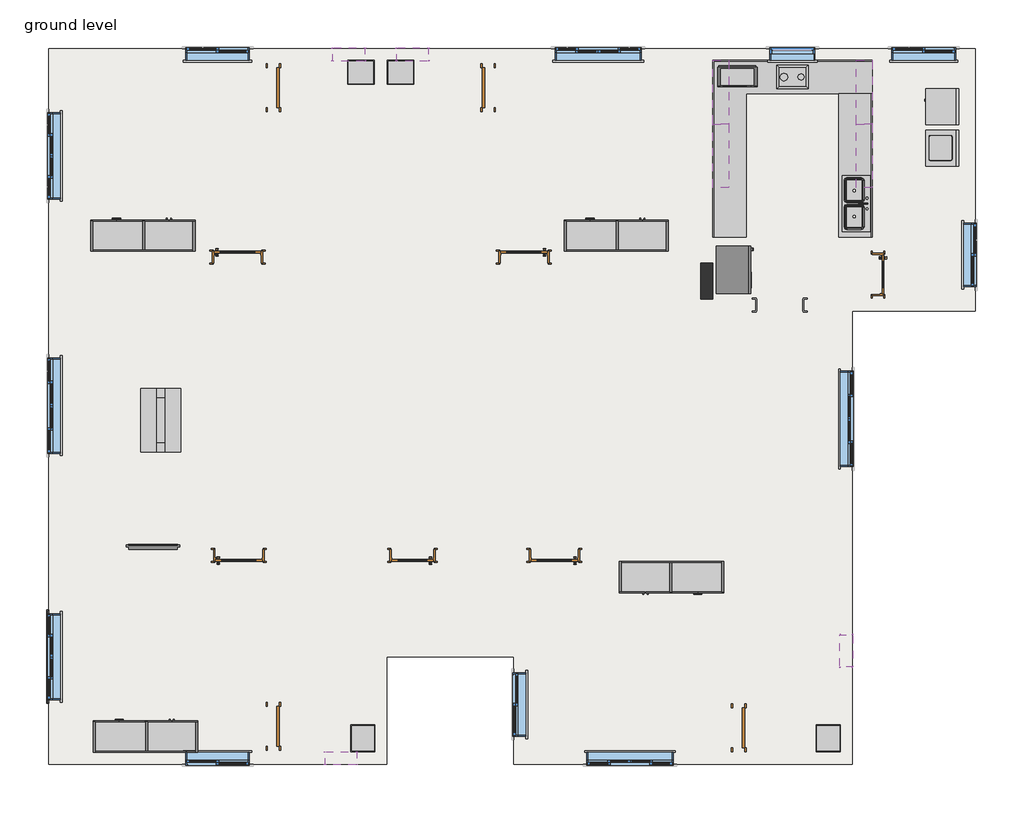
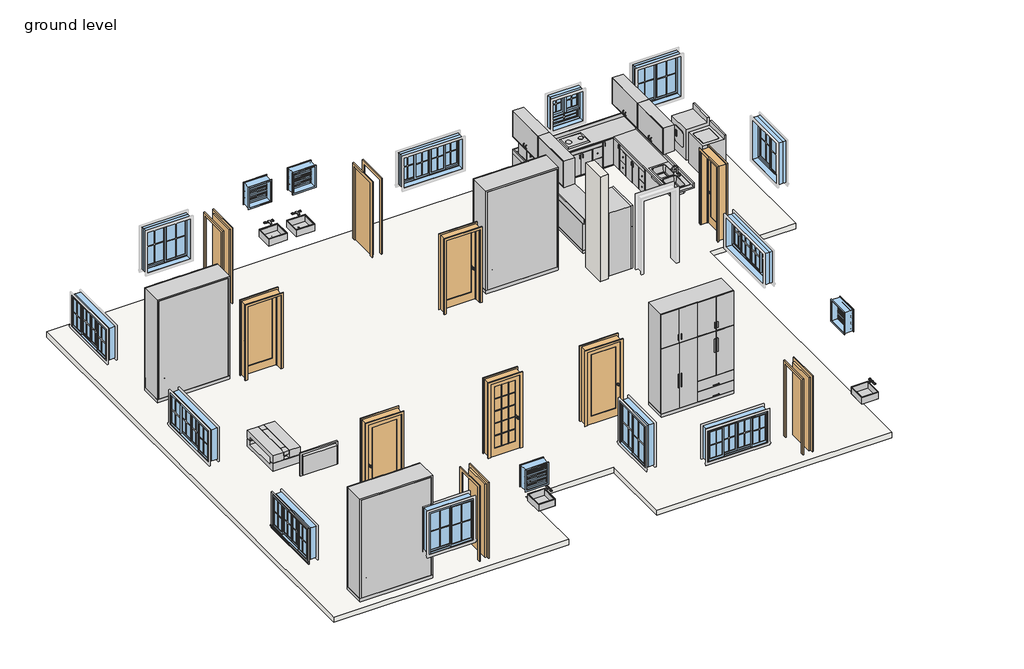
# One storey, part 1 of 2: 19 furniture elements, 16 windows, 10 doors, 10 proxies, 5 flow terminals, 1 slab, 1 wall.
"""IFC4 building model written with IfcOpenShell, lengths in millimetres."""

from ifc_helpers import new_model, si_unit, frame, origin, place, context, project, spatial, polyline, outline, extrude, transform, mapped, element, save
from components import proxy_3c1fa1d0, proxy_97c73763, proxy_e661f726, muntin_pattern_2x2_muntin_pattern_2x2_6186d23a, muntin_pattern_2x2_muntin_pattern_2x2_31a16349, muntin_pattern_2x2_muntin_pattern_2x2_cf37b409, trim_window_exterior_flat_with_sill_c3f87112, proxy_e75280ca, door_ac3c0746, door_868ee8a9, door_3b97b8e7, door_c0815308, door_5e1232af, door_bb98abfd, flow_terminal_cce4e9d2, flow_terminal_a53be723, furniture_65fa61b5, furniture_1wardrobe_6271_1wardrobe_6271_4dd35231, furniture_3428e43d, furniture_97fe820d, furniture_803bf5e8, furniture_2797bbf7, furniture_b6aab1a0, furniture_ea954fa4, white_modern_coffee_table_17067_white_modern_coffee_table_d4aed9ff, window_ced37e8f, window_f2d8fef0, window_5af5dca6, window_95c4569f, window_58cce754

model = new_model("IFC4")

# Units and contexts
model_context = context("Model", 3, world=origin())
ifc_project = project(units=[si_unit("LENGTHUNIT", "METRE", prefix="MILLI")], contexts=[model_context])

# Site, building, storey
site = spatial("IfcSite", under=ifc_project)
building = spatial("IfcBuilding", under=site)
storey = spatial("IfcBuildingStorey", under=building, Name="ground level", Elevation=609.6)

# Proxies
placement = place(None, origin())
proxy_shape = proxy_3c1fa1d0(model_context)
element("IfcBuildingElementProxy", 1, Name="Cook Top-2 Unit : 12\" x 18\" 2", ObjectType="Cook Top-2 Unit : 12\" x 18\" 2", at=placement, inside=storey, context=model_context, shape_type="MappedRepresentation", body=[
    mapped(proxy_shape, transform((6250.0508793, 6451.6660813, 609.6), x_axis=(0.0, 1.0, 0.0), y_axis=(-1.0, 0.0, 0.0), z_axis=(0.0, 0.0, 1.0))),
])
proxy_2_shape = proxy_97c73763(model_context)
element("IfcBuildingElementProxy", 2, Name="Dryer : 27\" x 25\" x 35\"", ObjectType="Dryer : 27\" x 25\" x 35\"", at=placement, inside=storey, context=model_context, shape_type="MappedRepresentation", body=[
    mapped(proxy_2_shape, transform((8776.0370876, 6339.378625, 609.6), x_axis=(0.0, -1.0, 0.0), y_axis=(1.0, 0.0, 0.0), z_axis=(0.0, 0.0, 1.0))),
])
proxy_3_shape = proxy_e661f726(model_context)
element("IfcBuildingElementProxy", 3, Name="Microwave : 30\" x 16\" x 18\"", ObjectType="Microwave : 30\" x 16\" x 18\"", at=placement, inside=storey, context=model_context, shape_type="MappedRepresentation", body=[
    mapped(proxy_3_shape, transform((4665.4332064, 6893.6465872, 609.6), x_axis=(1.0, 0.0, 0.0), y_axis=(0.0, 1.0, 0.0), z_axis=(0.0, 0.0, 1.0))),
])
muntin_pattern_2x2_muntin_pattern_2x2_shape = muntin_pattern_2x2_muntin_pattern_2x2_6186d23a(model_context)
element("IfcBuildingElementProxy", 4, Name="Muntin Pattern_2x2 : Muntin Pattern_2x2", ObjectType="Muntin Pattern_2x2 : Muntin Pattern_2x2", at=placement, inside=storey, context=model_context, shape_type="MappedRepresentation", body=[
    mapped(muntin_pattern_2x2_muntin_pattern_2x2_shape, transform((-8020.0489162, -5178.3589187, 1606.55), x_axis=(0.0, 1.0, 0.0), y_axis=(-1.0, 0.0, 0.0), z_axis=(0.0, 0.0, 1.0))),
])
element("IfcBuildingElementProxy", 5, Name="Muntin Pattern_2x2 : Muntin Pattern_2x2", ObjectType="Muntin Pattern_2x2 : Muntin Pattern_2x2", at=placement, inside=storey, context=model_context, shape_type="MappedRepresentation", body=[
    mapped(muntin_pattern_2x2_muntin_pattern_2x2_shape, transform((-8020.0489162, -3990.9089187, 1606.55), x_axis=(0.0, 1.0, 0.0), y_axis=(-1.0, 0.0, 0.0), z_axis=(0.0, 0.0, 1.0))),
])
muntin_pattern_2x2_muntin_pattern_2x2_2_shape = muntin_pattern_2x2_muntin_pattern_2x2_31a16349(model_context)
element("IfcBuildingElementProxy", 6, Name="Muntin Pattern_2x2 : Muntin Pattern_2x2", ObjectType="Muntin Pattern_2x2 : Muntin Pattern_2x2", at=placement, inside=storey, context=model_context, shape_type="MappedRepresentation", body=[
    mapped(muntin_pattern_2x2_muntin_pattern_2x2_2_shape, transform((-8020.0489162, -431.7339187, 1606.55), x_axis=(0.0, 1.0, 0.0), y_axis=(-1.0, 0.0, 0.0), z_axis=(0.0, 0.0, 1.0))),
])
muntin_pattern_2x2_muntin_pattern_2x2_3_shape = muntin_pattern_2x2_muntin_pattern_2x2_cf37b409(model_context)
element("IfcBuildingElementProxy", 7, Name="Muntin Pattern_2x2 : Muntin Pattern_2x2", ObjectType="Muntin Pattern_2x2 : Muntin Pattern_2x2", at=placement, inside=storey, context=model_context, shape_type="MappedRepresentation", body=[
    mapped(muntin_pattern_2x2_muntin_pattern_2x2_3_shape, transform((-5075.2364162, -6588.0589187, 1606.55), x_axis=(-1.0, 0.0, 0.0), y_axis=(0.0, -1.0, 0.0), z_axis=(0.0, 0.0, 1.0))),
])
element("IfcBuildingElementProxy", 8, Name="Muntin Pattern_2x2 : Muntin Pattern_2x2", ObjectType="Muntin Pattern_2x2 : Muntin Pattern_2x2", at=placement, inside=storey, context=model_context, shape_type="MappedRepresentation", body=[
    mapped(muntin_pattern_2x2_muntin_pattern_2x2_3_shape, transform((-4506.9114162, -6632.5089187, 1606.55), x_axis=(-1.0, 0.0, 0.0), y_axis=(0.0, -1.0, 0.0), z_axis=(0.0, 0.0, 1.0))),
])
trim_window_exterior_flat_with_sill_shape = trim_window_exterior_flat_with_sill_c3f87112(model_context)
element("IfcBuildingElementProxy", 9, Name="Trim-Window-Exterior-Flat : with Sill", ObjectType="Trim-Window-Exterior-Flat : with Sill", at=placement, inside=storey, context=model_context, shape_type="MappedRepresentation", body=[
    mapped(trim_window_exterior_flat_with_sill_shape, transform((-8029.5739162, -4584.6339187, 2438.4), x_axis=(0.0, -1.0, 0.0), y_axis=(0.0, 0.0, 1.0), z_axis=(-1.0, 0.0, 0.0))),
])
proxy_4_shape = proxy_e75280ca(model_context)
element("IfcBuildingElementProxy", 10, Name="Washer : 27\" x 25\" x 35\"", ObjectType="Washer : 27\" x 25\" x 35\"", at=placement, inside=storey, context=model_context, shape_type="MappedRepresentation", body=[
    mapped(proxy_4_shape, transform((8810.3756486, 5586.7486128, 609.6), x_axis=(0.0, -1.0, 0.0), y_axis=(1.0, 0.0, 0.0), z_axis=(0.0, 0.0, 1.0))),
])

# Doors
door_shape = door_ac3c0746(model_context)
element("IfcDoor", 11, ObjectType="Door-Interior-Single-1_Panel-Wood : 30\" x 84\"", at=placement, inside=storey, context=model_context, shape_type="MappedRepresentation", body=[
    mapped(door_shape, transform((7861.3010838, 2743.2660813, 609.6), x_axis=(0.0, -1.0, 0.0), y_axis=(1.0, 0.0, 0.0), z_axis=(0.0, 0.0, 1.0))),
])
door_2_shape = door_868ee8a9(model_context)
element("IfcDoor", 12, ObjectType="Door-Interior-Single-1_Panel-Wood : 36\" x 84\"", at=placement, inside=storey, context=model_context, shape_type="MappedRepresentation", body=[
    mapped(door_2_shape, transform((1076.3260838, 3076.6410813, 609.6), x_axis=(-1.0, 0.0, 0.0), y_axis=(0.0, -1.0, 0.0), z_axis=(0.0, 0.0, 1.0))),
])
element("IfcDoor", 13, ObjectType="Door-Interior-Single-1_Panel-Wood : 36\" x 84\"", at=placement, inside=storey, context=model_context, shape_type="MappedRepresentation", body=[
    mapped(door_2_shape, transform((-4384.6739162, -2644.7089187, 609.6), x_axis=(1.0, 0.0, 0.0), y_axis=(0.0, 1.0, 0.0), z_axis=(0.0, 0.0, 1.0))),
])
door_3_shape = door_3b97b8e7(model_context)
element("IfcDoor", 14, ObjectType="Door-Interior-Single-1_Panel-Wood : 36\" x 84\"", at=placement, inside=storey, context=model_context, shape_type="MappedRepresentation", body=[
    mapped(door_3_shape, transform((1660.5260838, -2644.7089187, 609.6), x_axis=(-1.0, 0.0, 0.0), y_axis=(0.0, -1.0, 0.0), z_axis=(0.0, 0.0, 1.0))),
])
element("IfcDoor", 15, ObjectType="Door-Interior-Single-1_Panel-Wood : 36\" x 84\"", at=placement, inside=storey, context=model_context, shape_type="MappedRepresentation", body=[
    mapped(door_3_shape, transform((-4410.0739162, 3076.6410813, 609.6), x_axis=(1.0, 0.0, 0.0), y_axis=(0.0, 1.0, 0.0), z_axis=(0.0, 0.0, 1.0))),
])
door_4_shape = door_c0815308(model_context)
element("IfcDoor", 16, ObjectType="Door-Interior-Single-Full Glass-Wood : 32\" x 84\"", at=placement, inside=storey, context=model_context, shape_type="MappedRepresentation", body=[
    mapped(door_4_shape, transform((-1057.2739162, -2644.7089187, 609.6), x_axis=(-1.0, 0.0, 0.0), y_axis=(0.0, -1.0, 0.0), z_axis=(0.0, 0.0, 1.0))),
])
door_5_shape = door_5e1232af(model_context)
element("IfcDoor", 17, ObjectType="Single-Flush : 30\" x 84\"", at=placement, inside=storey, context=model_context, shape_type="MappedRepresentation", body=[
    mapped(door_5_shape, transform((-3724.2739162, 6324.6660813, 609.6), x_axis=(0.0, 1.0, 0.0), y_axis=(-1.0, 0.0, 0.0), z_axis=(0.0, 0.0, 1.0))),
])
door_6_shape = door_bb98abfd(model_context)
element("IfcDoor", 18, ObjectType="Single-Flush : 30\" x 84\"", at=placement, inside=storey, context=model_context, shape_type="MappedRepresentation", body=[
    mapped(door_6_shape, transform((390.5260838, 6324.6660813, 609.6), x_axis=(0.0, 1.0, 0.0), y_axis=(-1.0, 0.0, 0.0), z_axis=(0.0, 0.0, 1.0))),
])
element("IfcDoor", 19, ObjectType="Single-Flush : 30\" x 84\"", at=placement, inside=storey, context=model_context, shape_type="MappedRepresentation", body=[
    mapped(door_6_shape, transform((-3724.2739162, -5918.1339187, 609.6), x_axis=(0.0, -1.0, 0.0), y_axis=(1.0, 0.0, 0.0), z_axis=(0.0, 0.0, 1.0))),
])
element("IfcDoor", 20, ObjectType="Single-Flush : 30\" x 84\"", at=placement, inside=storey, context=model_context, shape_type="MappedRepresentation", body=[
    mapped(door_6_shape, transform((5191.1260838, -5943.5339187, 609.6), x_axis=(0.0, -1.0, 0.0), y_axis=(1.0, 0.0, 0.0), z_axis=(0.0, 0.0, 1.0))),
])

# Flow terminals
flow_terminal_shape = flow_terminal_cce4e9d2(model_context)
element("IfcFlowTerminal", 21, ObjectType="Sink - Work : 20\"x18\"", at=placement, inside=storey, context=model_context, shape_type="MappedRepresentation", body=[
    mapped(flow_terminal_shape, transform((-1285.8739162, 6845.3660813, 1524.0), x_axis=(1.0, 0.0, 0.0), y_axis=(0.0, 1.0, 0.0), z_axis=(0.0, 0.0, 1.0))),
])
element("IfcFlowTerminal", 22, ObjectType="Sink - Work : 20\"x18\"", at=placement, inside=storey, context=model_context, shape_type="MappedRepresentation", body=[
    mapped(flow_terminal_shape, transform((-2047.8739162, 6845.3660813, 1524.0), x_axis=(1.0, 0.0, 0.0), y_axis=(0.0, 1.0, 0.0), z_axis=(0.0, 0.0, 1.0))),
])
element("IfcFlowTerminal", 23, ObjectType="Sink - Work : 20\"x18\"", at=placement, inside=storey, context=model_context, shape_type="MappedRepresentation", body=[
    mapped(flow_terminal_shape, transform((-1781.1739162, -6146.7339187, 1524.0), x_axis=(0.0, -1.0, 0.0), y_axis=(1.0, 0.0, 0.0), z_axis=(0.0, 0.0, 1.0))),
])
element("IfcFlowTerminal", 24, ObjectType="Sink - Work : 20\"x18\"", at=placement, inside=storey, context=model_context, shape_type="MappedRepresentation", body=[
    mapped(flow_terminal_shape, transform((7134.2260838, -6146.7339187, 1524.0), x_axis=(0.0, -1.0, 0.0), y_axis=(1.0, 0.0, 0.0), z_axis=(0.0, 0.0, 1.0))),
])
flow_terminal_2_shape = flow_terminal_a53be723(model_context)
element("IfcFlowTerminal", 25, ObjectType="Sink Kitchen-Double : 42\" x 21\"", at=placement, inside=storey, context=model_context, shape_type="MappedRepresentation", body=[
    mapped(flow_terminal_2_shape, transform((7436.6806826, 4117.8553219, 609.6), x_axis=(0.0, -1.0, 0.0), y_axis=(1.0, 0.0, 0.0), z_axis=(0.0, 0.0, 1.0))),
])

# Furniture
furniture_shape = furniture_65fa61b5(model_context)
element("IfcFurniture", 26, at=placement, inside=storey, context=model_context, shape_type="MappedRepresentation", body=[
    mapped(furniture_shape, transform((4759.3260838, 3441.7660813, 609.6), x_axis=(0.0, 1.0, 0.0), y_axis=(-1.0, 0.0, 0.0), z_axis=(0.0, 0.0, 1.0))),
])
furniture_1wardrobe_6271_1wardrobe_6271_shape = furniture_1wardrobe_6271_1wardrobe_6271_4dd35231(model_context)
element("IfcFurniture", 27, ObjectType="1Wardrobe_6271 : 1Wardrobe_6271", at=placement, inside=storey, context=model_context, shape_type="MappedRepresentation", body=[
    mapped(furniture_1wardrobe_6271_1wardrobe_6271_shape, transform((-5222.8739162, 3187.7660813, 609.6), x_axis=(-1.0, 0.0, 0.0), y_axis=(0.0, -1.0, 0.0), z_axis=(0.0, 0.0, 1.0))),
])
element("IfcFurniture", 28, ObjectType="1Wardrobe_6271 : 1Wardrobe_6271", at=placement, inside=storey, context=model_context, shape_type="MappedRepresentation", body=[
    mapped(furniture_1wardrobe_6271_1wardrobe_6271_shape, transform((3844.9260838, 3187.7660813, 609.6), x_axis=(-1.0, 0.0, 0.0), y_axis=(0.0, -1.0, 0.0), z_axis=(0.0, 0.0, 1.0))),
])
element("IfcFurniture", 29, ObjectType="1Wardrobe_6271 : 1Wardrobe_6271", at=placement, inside=storey, context=model_context, shape_type="MappedRepresentation", body=[
    mapped(furniture_1wardrobe_6271_1wardrobe_6271_shape, transform((2905.1260838, -2755.8339187, 609.6), x_axis=(1.0, 0.0, 0.0), y_axis=(0.0, 1.0, 0.0), z_axis=(0.0, 0.0, 1.0))),
])
element("IfcFurniture", 30, ObjectType="1Wardrobe_6271 : 1Wardrobe_6271", at=placement, inside=storey, context=model_context, shape_type="MappedRepresentation", body=[
    mapped(furniture_1wardrobe_6271_1wardrobe_6271_shape, transform((-5172.0739162, -6413.4339187, 609.6), x_axis=(-1.0, 0.0, 0.0), y_axis=(0.0, -1.0, 0.0), z_axis=(0.0, 0.0, 1.0))),
])
furniture_2_shape = furniture_3428e43d(model_context)
element("IfcFurniture", 31, ObjectType="48\" 2", at=placement, inside=storey, context=model_context, shape_type="MappedRepresentation", body=[
    mapped(furniture_2_shape, transform((6128.9811238, 6845.3660813, 609.6), x_axis=(1.0, 0.0, 0.0), y_axis=(0.0, 1.0, 0.0), z_axis=(0.0, 0.0, 1.0))),
])
element("IfcFurniture", 32, ObjectType="48\" 2", at=placement, inside=storey, context=model_context, shape_type="MappedRepresentation", body=[
    mapped(furniture_2_shape, transform((7743.8260838, 5412.2110413, 609.6), x_axis=(0.0, -1.0, 0.0), y_axis=(1.0, 0.0, 0.0), z_axis=(0.0, 0.0, 1.0))),
])
element("IfcFurniture", 33, ObjectType="48\" 2", at=placement, inside=storey, context=model_context, shape_type="MappedRepresentation", body=[
    mapped(furniture_2_shape, transform((4695.8260838, 5230.5211213, 609.6), x_axis=(0.0, 1.0, 0.0), y_axis=(-1.0, 0.0, 0.0), z_axis=(0.0, 0.0, 1.0))),
])
element("IfcFurniture", 34, ObjectType="48\" 2", at=placement, inside=storey, context=model_context, shape_type="MappedRepresentation", body=[
    mapped(furniture_2_shape, transform((4695.8260838, 4011.3211213, 609.6), x_axis=(0.0, 1.0, 0.0), y_axis=(-1.0, 0.0, 0.0), z_axis=(0.0, 0.0, 1.0))),
])
furniture_3_shape = furniture_97fe820d(model_context)
element("IfcFurniture", 35, ObjectType="Base Cabinet-Corner Unit-Square : 36\"", at=placement, inside=storey, context=model_context, shape_type="MappedRepresentation", body=[
    mapped(furniture_3_shape, transform((7217.0883788, 6845.3660813, 609.6), x_axis=(1.0, 0.0, 0.0), y_axis=(0.0, 1.0, 0.0), z_axis=(0.0, 0.0, 1.0))),
])
element("IfcFurniture", 36, ObjectType="Base Cabinet-Corner Unit-Square : 36\"", at=placement, inside=storey, context=model_context, shape_type="MappedRepresentation", body=[
    mapped(furniture_3_shape, transform((4695.8260838, 6318.6283764, 609.6), x_axis=(0.0, 1.0, 0.0), y_axis=(-1.0, 0.0, 0.0), z_axis=(0.0, 0.0, 1.0))),
])
furniture_4_shape = furniture_803bf5e8(model_context)
element("IfcFurniture", 37, ObjectType="Counter Top w Sink : 24\" Depth", at=placement, inside=storey, context=model_context, shape_type="MappedRepresentation", body=[
    mapped(furniture_4_shape, transform((7743.8260838, 5009.9037862, 609.6), x_axis=(0.0, -1.0, 0.0), y_axis=(1.0, 0.0, 0.0), z_axis=(0.0, 0.0, 1.0))),
])
furniture_5_shape = furniture_2797bbf7(model_context)
element("IfcFurniture", 38, ObjectType="Counter Top-L Shaped : 24\" Depth", at=placement, inside=storey, context=model_context, shape_type="MappedRepresentation", body=[
    mapped(furniture_5_shape, transform((5896.2883788, 6845.3660813, 609.6), x_axis=(1.0, 0.0, 0.0), y_axis=(0.0, 1.0, 0.0), z_axis=(0.0, 0.0, 1.0))),
])
furniture_6_shape = furniture_b6aab1a0(model_context)
element("IfcFurniture", 39, ObjectType="Television-Plasma : 42\"", at=placement, inside=storey, context=model_context, shape_type="MappedRepresentation", body=[
    mapped(furniture_6_shape, transform((-5972.1739162, -2527.2339187, 1676.4), x_axis=(-1.0, 0.0, 0.0), y_axis=(0.0, -1.0, 0.0), z_axis=(0.0, 0.0, 1.0))),
])
furniture_7_shape = furniture_ea954fa4(model_context)
element("IfcFurniture", 40, ObjectType="Upper Cabinet-Pass-Thru : 48\" x 30\" x 12\"", at=placement, inside=storey, context=model_context, shape_type="MappedRepresentation", body=[
    mapped(furniture_7_shape, transform((4695.8260838, 6217.0283764, 609.6), x_axis=(0.0, 1.0, 0.0), y_axis=(-1.0, 0.0, 0.0), z_axis=(0.0, 0.0, 1.0))),
])
element("IfcFurniture", 41, ObjectType="Upper Cabinet-Pass-Thru : 48\" x 30\" x 12\"", at=placement, inside=storey, context=model_context, shape_type="MappedRepresentation", body=[
    mapped(furniture_7_shape, transform((4695.8260838, 4997.8283764, 609.6), x_axis=(0.0, 1.0, 0.0), y_axis=(-1.0, 0.0, 0.0), z_axis=(0.0, 0.0, 1.0))),
])
element("IfcFurniture", 42, ObjectType="Upper Cabinet-Pass-Thru : 48\" x 30\" x 12\"", at=placement, inside=storey, context=model_context, shape_type="MappedRepresentation", body=[
    mapped(furniture_7_shape, transform((7743.8260838, 6254.5037862, 609.6), x_axis=(0.0, -1.0, 0.0), y_axis=(1.0, 0.0, 0.0), z_axis=(0.0, 0.0, 1.0))),
])
element("IfcFurniture", 43, ObjectType="Upper Cabinet-Pass-Thru : 48\" x 30\" x 12\"", at=placement, inside=storey, context=model_context, shape_type="MappedRepresentation", body=[
    mapped(furniture_7_shape, transform((7743.8260838, 5035.3037862, 609.6), x_axis=(0.0, -1.0, 0.0), y_axis=(1.0, 0.0, 0.0), z_axis=(0.0, 0.0, 1.0))),
])
white_modern_coffee_table_17067_white_modern_coffee_table_shape = white_modern_coffee_table_17067_white_modern_coffee_table_d4aed9ff(model_context)
element("IfcFurniture", 44, ObjectType="White_Modern_Coffee_Table_17067 : White_Modern_Coffee_Table_17067", at=placement, inside=storey, context=model_context, shape_type="MappedRepresentation", body=[
    mapped(white_modern_coffee_table_17067_white_modern_coffee_table_shape, transform((-5878.4127262, -50.7339187, 609.6), x_axis=(0.0, 1.0, 0.0), y_axis=(-1.0, 0.0, 0.0), z_axis=(0.0, 0.0, 1.0))),
])

# Slab
element("IfcSlab", 45, ObjectType="Generic - 6\"", at=placement, inside=storey, context=model_context, shape_type="SweptSolid", body=[
    extrude(outline(polyline([(9725.2894662, 7073.9660813), (9725.2894662, 2044.7660813), (7362.8260838, 2044.7660813), (7362.8260838, -6642.0339187), (885.8260838, -6642.0339187), (885.8260838, -4584.6339187), (-1552.5739162, -4584.6339187), (-1552.5739162, -6642.0339187), (-8029.5739162, -6642.0339187), (-8029.5739162, 7073.9660813), (9725.2894662, 7073.9660813)])), frame((0.0, 0.0, 457.2), z_axis=(0.0, 0.0, 1.0), x_axis=(1.0, 0.0, 0.0)), (0.0, 0.0, 1.0), 152.4),
])

# Wall
element("IfcWall", 46, ObjectType="Generic - 9\"", at=placement, inside=storey, context=model_context, shape_type="SweptSolid", body=[
    extrude(outline(polyline([(4695.8260838, 2959.1660813), (4695.8260838, 2273.3660813), (4467.2260838, 2273.3660813), (4467.2260838, 2959.1660813), (4695.8260838, 2959.1660813)])), frame((0.0, 0.0, 609.6), z_axis=(0.0, 0.0, 1.0), x_axis=(1.0, 0.0, 0.0)), (0.0, 0.0, 1.0), 3048.0),
])

# Windows
window_shape = window_ced37e8f(model_context)
element("IfcWindow", 47, ObjectType="Window-Casement-Double-Awning : 34\" x 36\"", at=placement, inside=storey, context=model_context, shape_type="MappedRepresentation", body=[
    mapped(window_shape, transform((6219.8260838, 6959.6660813, 838.2), x_axis=(1.0, 0.0, 0.0), y_axis=(0.0, 1.0, 0.0), z_axis=(0.0, 0.0, 1.0))),
])
window_2_shape = window_f2d8fef0(model_context)
element("IfcWindow", 48, ObjectType="Window-Louvers : 24\" x 24\"", at=placement, inside=storey, context=model_context, shape_type="MappedRepresentation", body=[
    mapped(window_2_shape, transform((-2276.4739162, 6966.0160813, 1524.0), x_axis=(1.0, 0.0, 0.0), y_axis=(0.0, 1.0, 0.0), z_axis=(0.0, 0.0, 1.0))),
])
element("IfcWindow", 49, ObjectType="Window-Louvers : 24\" x 24\"", at=placement, inside=storey, context=model_context, shape_type="MappedRepresentation", body=[
    mapped(window_2_shape, transform((-1057.2739162, 6966.0160813, 1524.0), x_axis=(1.0, 0.0, 0.0), y_axis=(0.0, 1.0, 0.0), z_axis=(0.0, 0.0, 1.0))),
])
element("IfcWindow", 50, ObjectType="Window-Louvers : 24\" x 24\"", at=placement, inside=storey, context=model_context, shape_type="MappedRepresentation", body=[
    mapped(window_2_shape, transform((-2428.8739162, -6534.0839187, 1524.0), x_axis=(-1.0, 0.0, 0.0), y_axis=(0.0, -1.0, 0.0), z_axis=(0.0, 0.0, 1.0))),
])
element("IfcWindow", 51, ObjectType="Window-Louvers : 24\" x 24\"", at=placement, inside=storey, context=model_context, shape_type="MappedRepresentation", body=[
    mapped(window_2_shape, transform((7254.8760838, -4470.3339187, 1524.0), x_axis=(0.0, -1.0, 0.0), y_axis=(1.0, 0.0, 0.0), z_axis=(0.0, 0.0, 1.0))),
])
window_3_shape = window_5af5dca6(model_context)
element("IfcWindow", 52, ObjectType="Window-Sliding-Double : 48\" x 48\"", at=placement, inside=storey, context=model_context, shape_type="MappedRepresentation", body=[
    mapped(window_3_shape, transform((996.3160838, -5499.0339187, 609.6), x_axis=(0.0, 1.0, 0.0), y_axis=(-1.0, 0.0, 0.0), z_axis=(0.0, 0.0, 1.0))),
])
element("IfcWindow", 53, ObjectType="Window-Sliding-Double : 48\" x 48\"", at=placement, inside=storey, context=model_context, shape_type="MappedRepresentation", body=[
    mapped(window_3_shape, transform((8734.4260838, 6963.4760813, 609.6), x_axis=(1.0, 0.0, 0.0), y_axis=(0.0, 1.0, 0.0), z_axis=(0.0, 0.0, 1.0))),
])
element("IfcWindow", 54, ObjectType="Window-Sliding-Double : 48\" x 48\"", at=placement, inside=storey, context=model_context, shape_type="MappedRepresentation", body=[
    mapped(window_3_shape, transform((9614.7994662, 3116.7811041, 609.6), x_axis=(0.0, -1.0, 0.0), y_axis=(1.0, 0.0, 0.0), z_axis=(0.0, 0.0, 1.0))),
])
element("IfcWindow", 55, ObjectType="Window-Sliding-Double : 48\" x 48\"", at=placement, inside=storey, context=model_context, shape_type="MappedRepresentation", body=[
    mapped(window_3_shape, transform((-4791.0739162, -6531.5439187, 609.6), x_axis=(-1.0, 0.0, 0.0), y_axis=(0.0, -1.0, 0.0), z_axis=(0.0, 0.0, 1.0))),
])
element("IfcWindow", 56, ObjectType="Window-Sliding-Double : 48\" x 48\"", at=placement, inside=storey, context=model_context, shape_type="MappedRepresentation", body=[
    mapped(window_3_shape, transform((-4791.0739162, 6963.4760813, 609.6), x_axis=(1.0, 0.0, 0.0), y_axis=(0.0, 1.0, 0.0), z_axis=(0.0, 0.0, 1.0))),
])
window_4_shape = window_95c4569f(model_context)
element("IfcWindow", 57, ObjectType="Window-Sliding-Four : 65\" x 36\"", at=placement, inside=storey, context=model_context, shape_type="MappedRepresentation", body=[
    mapped(window_4_shape, transform((2498.7260838, 6963.4760813, 609.6), x_axis=(1.0, 0.0, 0.0), y_axis=(0.0, 1.0, 0.0), z_axis=(0.0, 0.0, 1.0))),
])
element("IfcWindow", 58, ObjectType="Window-Sliding-Four : 65\" x 36\"", at=placement, inside=storey, context=model_context, shape_type="MappedRepresentation", body=[
    mapped(window_4_shape, transform((3108.3260838, -6531.5439187, 609.6), x_axis=(-1.0, 0.0, 0.0), y_axis=(0.0, -1.0, 0.0), z_axis=(0.0, 0.0, 1.0))),
])
element("IfcWindow", 59, ObjectType="Window-Sliding-Four : 65\" x 36\"", at=placement, inside=storey, context=model_context, shape_type="MappedRepresentation", body=[
    mapped(window_4_shape, transform((-7919.0839162, 5016.5660813, 609.6), x_axis=(0.0, 1.0, 0.0), y_axis=(-1.0, 0.0, 0.0), z_axis=(0.0, 0.0, 1.0))),
])
element("IfcWindow", 60, ObjectType="Window-Sliding-Four : 65\" x 36\"", at=placement, inside=storey, context=model_context, shape_type="MappedRepresentation", body=[
    mapped(window_4_shape, transform((-7919.0839162, -4584.6339187, 609.6), x_axis=(0.0, 1.0, 0.0), y_axis=(-1.0, 0.0, 0.0), z_axis=(0.0, 0.0, 1.0))),
])
window_5_shape = window_58cce754(model_context)
element("IfcWindow", 61, ObjectType="Window-Sliding-Four : 72\" x 36\"", at=placement, inside=storey, context=model_context, shape_type="MappedRepresentation", body=[
    mapped(window_5_shape, transform((-7919.0839162, 228.6660813, 609.6), x_axis=(0.0, 1.0, 0.0), y_axis=(-1.0, 0.0, 0.0), z_axis=(0.0, 0.0, 1.0))),
])
element("IfcWindow", 62, ObjectType="Window-Sliding-Four : 72\" x 36\"", at=placement, inside=storey, context=model_context, shape_type="MappedRepresentation", body=[
    mapped(window_5_shape, transform((7252.3360838, -25.3339187, 609.6), x_axis=(0.0, -1.0, 0.0), y_axis=(1.0, 0.0, 0.0), z_axis=(0.0, 0.0, 1.0))),
])

save(model, "model.ifc")

# Revit data of these elements
# Type "Cook Top-2 Unit : 12\" x 18\" 2"
#   Assembly Code = "E1090400"
#   Counter Height = 3' - 0"
#   Depth = 2' - 0"
#   Width = 1' - 6"
#   Burner Material = Metal - Chrome
#   Cooktop Material = Metal - Steel, Polished
#   Default Elevation = 0
# Type "Dryer : 27\" x 25\" x 35\""
#   Label = "D"
#   Assembly Code = "E1090400"
#   Depth = 2' - 1"
#   Height = 2' - 11"
#   Width = 2' - 3"
#   Dryer Material = Metal - Paint Finish - Ivory,Glossy
#   Default Elevation = 0
# Type "Microwave : 30\" x 16\" x 18\""
#   Assembly Code = "E1090400"
#   Depth = 1' - 4"
#   Height = 1' - 6"
#   Width = 2' - 6"
#   Microwave Material = Laminate - Ivory,Matte
#   Default Elevation = 0
# Type "Muntin Pattern_2x2 : Muntin Pattern_2x2"
#   Width [instance default] = 4' - 0"
#   Thickness = 0' - 0 1/2"
#   Height [instance default] = 4' - 0"
#   Distance = 0' - 0 3/4"
#   Interior Material [instance default] = none
#   Exterior Material [instance default] = none
#   Default Elevation = 0
# Type "Trim-Window-Exterior-Flat : with Sill"
#   Trim Width = 0' - 2 1/4"
#   Trim Thickness_Picture Frame = 0' - 1 1/4"
#   Trim Thickness_with Sill = 0' - 0 3/4"
#   Sill Thickness = 0' - 1 1/4"
#   Opening Width [instance default] = 2' - 0"
#   Opening Height [instance default] = 3' - 0"
#   Default Elevation = 4' - 0"
#   Sill = yes
#   Picture Frame = no
#   Trim Material [instance default] = none
# Type "Washer : 27\" x 25\" x 35\""
#   Label = "W"
#   Assembly Code = "E1090400"
#   Depth = 2' - 1"
#   Height = 2' - 11"
#   Width = 2' - 3"
#   Washer Material = Metal - Paint Finish - Ivory,Matte
#   Default Elevation = 0
# Type "Door-Interior-Single-1_Panel-Wood : 30\" x 84\""
#   Type Mark = "11"
#   Assembly Code = "C1020300"
#   Analytic Construction = "Wooden"
#   Top Rail = 0' - 4 11/16"
#   Thickness = 0' - 1 3/8"
#   Thermal Resistance (R) = 2.5876 (h·ft²·°F)/BTU
#   Swing Angle [instance default] = 90.00°
#   Stiles = 0' - 4 3/4"
#   Rough Width = 2' - 8"
#   Rough Height = 7' - 1"
#   Height = 7' - 0"
#   Width = 2' - 6"
#   Heat Transfer Coefficient (U) = 0.3865 BTU/(h·ft²·°F)
#   Bottom Rail = 0' - 9 1/8"
#   Trim Material = Cherry
#   Panel Material = Cherry
#   Frame Material = Cherry
#   Door Handle Material = Aluminum
#   Visual Light Transmittance = 0
#   Solar Heat Gain Coefficient = 0
#   Wall Closure = (empty or 0)
#   Function = (empty or 0)
# Type "Door-Interior-Single-1_Panel-Wood : 36\" x 84\""
#   Type Mark = "8"
#   Assembly Code = "C1020300"
#   Analytic Construction = "Wooden"
#   Top Rail = 0' - 4 11/16"
#   Thickness = 0' - 1 3/8"
#   Thermal Resistance (R) = 2.5876 (h·ft²·°F)/BTU
#   Swing Angle [instance default] = 90.00°
#   Stiles = 0' - 4 3/4"
#   Rough Width = 3' - 2"
#   Rough Height = 7' - 1"
#   Height = 7' - 0"
#   Width = 3' - 0"
#   Heat Transfer Coefficient (U) = 0.3865 BTU/(h·ft²·°F)
#   Bottom Rail = 0' - 9 1/8"
#   Trim Material = Cherry
#   Panel Material = Cherry
#   Frame Material = Cherry
#   Door Handle Material = Aluminum
#   Visual Light Transmittance = 0
#   Solar Heat Gain Coefficient = 0
#   Wall Closure = (empty or 0)
#   Function = (empty or 0)
# Type "Door-Interior-Single-Full Glass-Wood : 32\" x 84\""
#   Type Mark = "9"
#   Assembly Code = "C1020300"
#   Analytic Construction = "Wood frame with single clear glass"
#   Top Rail = 0' - 4 11/16"
#   Thickness = 0' - 1 3/8"
#   Thermal Resistance (R) = 1.0102 (h·ft²·°F)/BTU
#   Swing Angle [instance default] = 90.00°
#   Stiles = 0' - 4 3/4"
#   Rough Width = 2' - 10"
#   Rough Height = 7' - 1"
#   Height = 7' - 0"
#   Width = 2' - 8"
#   Heat Transfer Coefficient (U) = 0.9900 BTU/(h·ft²·°F)
#   Bottom Rail = 0' - 9 1/8"
#   Show Grill [instance default] = yes
#   Trim Material = Cherry
#   Panel Material = Cherry
#   Frame Material = Cherry
#   Door Handle Material = Aluminum
#   Visual Light Transmittance = 0
#   Solar Heat Gain Coefficient = 0
#   Wall Closure = (empty or 0)
#   Function = (empty or 0)
# Type "Single-Flush : 30\" x 84\""
#   Type Mark = "4"
#   Construction Type Id = "MDOOR"
#   Assembly Code = "C1020"
#   Analytic Construction = "Metal"
#   Thickness = 0' - 2"
#   Heat Transfer Coefficient (U) = 0.651978 BTU/(h·ft²·°F)
#   Height = 7' - 0"
#   Trim Projection Ext = 0' - 1"
#   Trim Projection Int = 0' - 1"
#   Trim Width = 0' - 3"
#   Width = 2' - 6"
#   Define Thermal Properties by = 1
#   Define Thermal Properties by = 1
#   Door Material = Door - Panel
#   Frame Material = Door - Frame
#   Visual Light Transmittance = 0
#   Solar Heat Gain Coefficient = 0
#   Function = (empty or 0)
#   Wall Closure = (empty or 0)
# Type "Sink - Work : 20\"x18\""
#   WFU = 2
#   Sink Width = 1' - 6"
#   Sink Length = 1' - 8"
#   Sink Depth = 0' - 8"
#   Sanitary Radius = 3/4"
#   Sanitary Diameter = 1 1/2"
#   Hot Water Radius = 1/4"
#   Hot Water Diameter = 1/2"
#   HWFU = 2.25
#   Flow Pressure [instance default] = 8.00 psi
#   Faucet Height = 1' - 1 5/8"
#   Cold Water Radius = 1/4"
#   Cold Water Diameter = 1/2"
#   CWFU = 2.25
#   Sink Material = none
#   Faucet Material = none
#   Default Elevation = 0
# Type "Sink Kitchen-Double : 42\" x 21\""
#   Assembly Code = "D2010410"
#   Counter Height = 3' - 0"
#   Depth = 1' - 9"
#   Width = 3' - 6"
#   Faucet Material = Steel, Polished
#   Sink Material = Steel, Polished
#   Default Elevation = 0
# Type
#   Default Elevation = 0
# Type "1Wardrobe_6271 : 1Wardrobe_6271"
#   Default Elevation = 0
# Type "48\" 2"
#   Assembly Code = "C1030410"
#   Depth = 2' - 0"
#   Height = 2' - 10 1/2"
#   Toe Depth = 0' - 3"
#   Toe Height = 0' - 3 1/2"
#   Width = 4' - 0"
#   Cabinet Material = none
#   Door/Drawer Material = none
#   Handle Material = Cabinets - Handles
#   Default Elevation = 0
# Type "Base Cabinet-Corner Unit-Square : 36\""
#   Assembly Code = "C1030410"
#   Depth = 2' - 0"
#   Height = 2' - 10 1/2"
#   Toe Depth = 0' - 3"
#   Toe Height = 0' - 3 1/2"
#   Width = 3' - 0"
#   Cabinet Material = Cabinets
#   Door/Drawer Material = Cabinets
#   Handle Material = Cabinets - Handles
#   Default Elevation = 0
# Type "Counter Top w Sink : 24\" Depth"
#   Assembly Code = "C1030400"
#   Counter Thickness = 0' - 1 1/2"
#   Depth = 2' - 1"
#   Height = 3' - 0"
#   Length [instance default] = 8' - 0"
#   Sink Location [instance default] = 2' - 0"
#   Sink Location To Wall [instance default] = 0' - 6"
#   Sink Opening Depth [instance default] = 1' - 3"
#   Sink Opening Width [instance default] = 3' - 3"
#   Counter Top Material = none
#   Default Elevation = 0
# Type "Counter Top-L Shaped : 24\" Depth"
#   Assembly Code = "C1030400"
#   Counter Thickness = 0' - 1 1/2"
#   Depth = 2' - 1"
#   Height = 3' - 0"
#   Length - Leg 1 [instance default] = 8' - 0"
#   Length - Leg 2 [instance default] = 6' - 0"
#   Counter Top Material = none
#   Default Elevation = 0
# Type "Television-Plasma : 42\""
#   Assembly Code = "E2020200"
#   Depth = 0' - 3 1/2"
#   Height = 2' - 2"
#   Width = 3' - 4 1/2"
#   Cabinet Material = Plastic - Gray
#   Default Elevation = 0
# Type "Upper Cabinet-Pass-Thru : 48\" x 30\" x 12\""
#   Depth = 1' - 0"
#   Height = 2' - 6"
#   Top of Cabinet = 7' - 0"
#   Width = 4' - 0"
#   Default Elevation = 0
# Type "White_Modern_Coffee_Table_17067 : White_Modern_Coffee_Table_17067"
#   White Modern Coffee Table - Wood Width = 0' - 6"
#   White Modern Coffee Table - Width = 2' - 6"
#   White Modern Coffee Table - Length = 4' - 0"
#   White Modern Coffee Table - Wood = White Modern Coffee Table - Wood
#   White Modern Coffee Table - Plastic = White Modern Coffee Table - Plastic
#   Default Elevation = 0
# Type "Generic - 6\""
#   Assembly Code = "B1010"
#   Function = 0
#   Layers, outside or top first: 0' - 6" no material (function 1)
# Type "Generic - 9\""
#   Assembly Code = "B2010"
#   Layers, outside or top first: 0' - 9" no material (function 1)
# Type "Window-Casement-Double-Awning : 34\" x 36\""
#   Type Mark = "26"
#   Fire Rating = "0.5h"
#   Assembly Code = "B2020100"
#   Analytic Construction = "Double glazing - domestic"
#   Window Inset [instance default] = 0' - 0"
#   Wall Thickness [instance default] = 0' - 6"
#   Interior Wall Closure [instance default] = 0' - 2 1/4"
#   Half Width = 1' - 5"
#   Visual Light Transmittance = 0.81
#   Thermal Resistance (R) = 1.8146 (h·ft²·°F)/BTU
#   Solar Heat Gain Coefficient = 0.76
#   Rough Width = 2' - 10 1/2"
#   Rough Height = 3' - 0 1/2"
#   Open Window Height = 2' - 0"
#   Height = 3' - 0"
#   Heat Transfer Coefficient (U) = 0.5511 BTU/(h·ft²·°F)
#   Frame Extension [instance default] = 0' - 0 1/4"
#   Exterior Wall Closure [instance default] = 0' - 1 1/4"
#   Awning Height = 1' - 0"
#   Extension Jamb [instance default] = 0' - 2 1/4"
#   Default Sill Height = 3' - 0"
#   Width = 2' - 10"
#   Top Muntin Visibility = yes
#   Interior Trim Visibility [instance default] = yes
#   Bottom Muntin Visibility = yes
#   Exterior Trim Visibility [instance default] = yes
#   Extension Jamb Visibility [instance default] = yes
#   Interior Trim Material = Wood - Stained
#   Muntin Pattern = Muntin Pattern_2x2 : Muntin Pattern_2x2
#   Interior Trim = Trim-Window-Interior-Flat : Picture Frame
#   Interior Frame Material = Wood - Stained
#   Exterior Trim Material = Clad - White
#   Glass Panel Material = Glass
#   Exterior Trim = Trim-Window-Exterior-Flat : with Sill
#   Exterior Frame Material = Clad - White
#   Wall Closure = (empty or 0)
# Type "Window-Louvers : 24\" x 24\""
#   Type Mark = "24"
#   Construction Type Id = "GSP4R"
#   Assembly Code = "B20"
#   Analytic Construction = "1/8 in Pilkington single glazing"
#   Visual Light Transmittance = 0.9
#   Thermal Resistance (R) = 1.53941 (h·ft²·°F)/BTU
#   Solar Heat Gain Coefficient = 0.78
#   Max Height = 1' - 11.74264"
#   Height = 2' - 0"
#   Heat Transfer Coefficient (U) = 0.6496 BTU/(h·ft²·°F)
#   Blade Width [instance default] = 1' - 10 1/2"
#   Blade Vertical Thickness = 0' - 0.35355"
#   Blade Thickness = 0' - 0 1/4"
#   Blade Spacing = 0' - 1 1/2"
#   Blade Height = 0' - 1.85355"
#   Blade Depth = 0' - 3"
#   Blade Angle = 45.00°
#   Default Sill Height = 3' - 0"
#   Trim Projection_Exterior = 0' - 0 1/2"
#   Trim Projection_Interior = 0' - 0 1/2"
#   Trim Width_Exterior = 0' - 1 1/2"
#   Trim Width_Interior = 0' - 1 1/2"
#   Width = 2' - 0"
#   Max Blade Count = 12
#   Define Thermal Properties by = 1
#   Blade Count = 12
#   Frame Material = Birch
#   Louver Material = Birch
#   Trim Exterior Material = Birch
#   Trim Interior Material = Birch
#   Wall Closure = (empty or 0)
# Type "Window-Sliding-Double : 48\" x 48\""
#   Type Mark = "23"
#   Fire Rating = "0.5h"
#   Assembly Code = "B2020100"
#   Analytic Construction = "Double glazing - domestic"
#   Window Inset [instance default] = 0' - 0"
#   Wall Thickness [instance default] = 0' - 6"
#   Visual Light Transmittance = 0.81
#   Thermal Resistance (R) = 1.8146 (h·ft²·°F)/BTU
#   Solar Heat Gain Coefficient = 0.76
#   Muntin Width = 1' - 8 5/8"
#   Muntin Height = 3' - 6 1/4"
#   Interior Wall Closure [instance default] = 0' - 2 3/4"
#   Heat Transfer Coefficient (U) = 0.5511 BTU/(h·ft²·°F)
#   Frame Extension [instance default] = 0' - 0 1/4"
#   Exterior Wall Closure [instance default] = 0' - 1 1/4"
#   Rough Width = 4' - 0 1/2"
#   Rough Height = 4' - 0 1/2"
#   Height = 4' - 0"
#   Extension Jamb [instance default] = 0' - 2 3/4"
#   Default Sill Height = 3' - 0"
#   Width = 4' - 0"
#   Interior Trim Visibility [instance default] = yes
#   Indicator Visibility [instance default] = yes
#   Exterior Trim Visibility [instance default] = yes
#   Muntin Visibility = yes
#   Extension Jamb Visibility [instance default] = yes
#   Muntin Pattern = Muntin Pattern_2x2 : Muntin Pattern_2x2
#   Interior Trim Material = Wood - Stained
#   Interior Trim = Trim-Window-Interior-Flat : Picture Frame
#   Interior Frame Material = Wood - Stained
#   Glass Panel Material = Glass
#   Exterior Trim Material = Clad - White
#   Exterior Trim = Trim-Window-Exterior-Flat : with Sill
#   Exterior Frame Material = Clad - White
#   Wall Closure = (empty or 0)
# Type "Window-Sliding-Four : 65\" x 36\""
#   Type Mark = "19"
#   Fire Rating = "0.5h"
#   Assembly Code = "B2020100"
#   Analytic Construction = "Double glazing - domestic"
#   Window Inset [instance default] = 0' - 0"
#   Wall Thickness [instance default] = 0' - 6"
#   Visual Light Transmittance = 0.81
#   Thermal Resistance (R) = 1.8146 (h·ft²·°F)/BTU
#   Solar Heat Gain Coefficient = 0.76
#   Interior Wall Closure [instance default] = 0' - 2 19/32"
#   Heat Transfer Coefficient (U) = 0.5511 BTU/(h·ft²·°F)
#   Frame Extension [instance default] = 0' - 0 1/4"
#   Exterior Wall Closure [instance default] = 0' - 1 1/4"
#   Rough Width = 5' - 5 1/2"
#   Rough Height = 3' - 0 1/2"
#   Height = 3' - 0"
#   Extension Jamb [instance default] = 0' - 2 3/4"
#   Default Sill Height = 3' - 0"
#   Width = 5' - 5"
#   Middle Muntin Visibility = yes
#   Interior Trim Visibility [instance default] = yes
#   Indicator Visibility [instance default] = yes
#   Exterior Trim Visibility [instance default] = yes
#   Side Muntin Visibility = yes
#   Extension Jamb Visibility [instance default] = yes
#   Interior Trim Material = Wood - Stained
#   Muntin Pattern = Muntin Pattern_2x2 : Muntin Pattern_2x2
#   Interior Trim = Trim-Window-Interior-Flat : Picture Frame
#   Interior Frame Material = Wood - Stained
#   Glass Panel Material = Glass
#   Exterior Trim Material = Clad - White
#   Exterior Trim = Trim-Window-Exterior-Flat : with Sill
#   Exterior Frame Material = Clad - White
#   Wall Closure = (empty or 0)
# Type "Window-Sliding-Four : 72\" x 36\""
#   Type Mark = "20"
#   Fire Rating = "0.5h"
#   Assembly Code = "B2020100"
#   Analytic Construction = "Double glazing - domestic"
#   Window Inset [instance default] = 0' - 0"
#   Wall Thickness [instance default] = 0' - 6"
#   Visual Light Transmittance = 0.81
#   Thermal Resistance (R) = 1.8146 (h·ft²·°F)/BTU
#   Solar Heat Gain Coefficient = 0.76
#   Interior Wall Closure [instance default] = 0' - 2 19/32"
#   Heat Transfer Coefficient (U) = 0.5511 BTU/(h·ft²·°F)
#   Frame Extension [instance default] = 0' - 0 1/4"
#   Exterior Wall Closure [instance default] = 0' - 1 1/4"
#   Rough Width = 6' - 0 1/2"
#   Rough Height = 3' - 0 1/2"
#   Height = 3' - 0"
#   Extension Jamb [instance default] = 0' - 2 3/4"
#   Default Sill Height = 3' - 0"
#   Width = 6' - 0"
#   Middle Muntin Visibility = yes
#   Interior Trim Visibility [instance default] = yes
#   Indicator Visibility [instance default] = yes
#   Exterior Trim Visibility [instance default] = yes
#   Side Muntin Visibility = yes
#   Extension Jamb Visibility [instance default] = yes
#   Interior Trim Material = Wood - Stained
#   Muntin Pattern = Muntin Pattern_2x2 : Muntin Pattern_2x2
#   Interior Trim = Trim-Window-Interior-Flat : Picture Frame
#   Interior Frame Material = Wood - Stained
#   Glass Panel Material = Glass
#   Exterior Trim Material = Clad - White
#   Exterior Trim = Trim-Window-Exterior-Flat : with Sill
#   Exterior Frame Material = Clad - White
#   Wall Closure = (empty or 0)
# Element 1 (IfcBuildingElementProxy, "Cook Top-2 Unit : 12\" x 18\" 2")
#   Phase Created = New Construction
#   Materials on its faces: "Metal - Steel, Polished", "Metal - Chrome"
# Element 2 (IfcBuildingElementProxy, "Dryer : 27\" x 25\" x 35\"")
#   Phase Created = New Construction
#   Materials on its faces: "Metal - Paint Finish - Ivory,Glossy"
# Element 3 (IfcBuildingElementProxy, "Microwave : 30\" x 16\" x 18\"")
#   Phase Created = New Construction
#   Materials on its faces: "Laminate - Ivory,Matte", "Glass"
# Elements 4, 5 (IfcBuildingElementProxy, "Muntin Pattern_2x2 : Muntin Pattern_2x2")
#   Width = 1' - 1 1/4"
#   Height = 2' - 6 1/4"
#   Interior Material = Wood - Stained
#   Exterior Material = Clad - White
#   Phase Created = New Construction
#   Materials on its faces: "Clad - White", "Wood - Stained"
# Element 6 (IfcBuildingElementProxy, "Muntin Pattern_2x2 : Muntin Pattern_2x2")
#   Width = 1' - 3"
#   Height = 2' - 6 1/4"
#   Interior Material = Wood - Stained
#   Exterior Material = Clad - White
#   Phase Created = New Construction
#   Materials on its faces: "Clad - White", "Wood - Stained"
# Elements 7, 8 (IfcBuildingElementProxy, "Muntin Pattern_2x2 : Muntin Pattern_2x2")
#   Width = 1' - 8 5/8"
#   Height = 3' - 6 1/4"
#   Interior Material = Wood - Stained
#   Exterior Material = Clad - White
#   Phase Created = New Construction
#   Materials on its faces: "Clad - White", "Wood - Stained"
# Element 9 (IfcBuildingElementProxy, "Trim-Window-Exterior-Flat : with Sill")
#   Opening Width = 5' - 5"
#   Opening Height = 3' - 0"
#   Trim Material = Clad - White
#   Phase Created = New Construction
#   Materials on its faces: "Clad - White"
# Element 10 (IfcBuildingElementProxy, "Washer : 27\" x 25\" x 35\"")
#   Phase Created = New Construction
#   Materials on its faces: "Metal - Paint Finish - Ivory,Matte"
# Element 11 (IfcDoor, "Door-Interior-Single-1_Panel-Wood : 30\" x 84\"")
#   Swing Angle = 90.00°
#   Phase Created = New Construction
#   Materials on its faces: "Cherry", "Aluminum"
# Elements 12, 13, 14, 15 (IfcDoor, "Door-Interior-Single-1_Panel-Wood : 36\" x 84\"")
#   Swing Angle = 90.00°
#   Phase Created = New Construction
#   Materials on its faces: "Cherry", "Aluminum"
# Element 16 (IfcDoor, "Door-Interior-Single-Full Glass-Wood : 32\" x 84\"")
#   Swing Angle = 90.00°
#   Show Grill = yes
#   Phase Created = New Construction
#   Materials on its faces: "Cherry", "Aluminum", "Glass"
# Elements 17, 18, 19, 20 (IfcDoor, "Single-Flush : 30\" x 84\"")
#   Phase Created = New Construction
#   Materials on its faces: "Door - Frame", "Door - Panel"
# Element 21 (IfcFlowTerminal, "Sink - Work : 20\"x18\"")
#   Mark = "6"
#   Flow Pressure = 8.00 psi
#   Phase Created = New Construction
# Element 22 (IfcFlowTerminal, "Sink - Work : 20\"x18\"")
#   Mark = "7"
#   Flow Pressure = 8.00 psi
#   Phase Created = New Construction
# Element 23 (IfcFlowTerminal, "Sink - Work : 20\"x18\"")
#   Mark = "8"
#   Flow Pressure = 8.00 psi
#   Phase Created = New Construction
# Element 24 (IfcFlowTerminal, "Sink - Work : 20\"x18\"")
#   Mark = "9"
#   Flow Pressure = 8.00 psi
#   Phase Created = New Construction
# Element 25 (IfcFlowTerminal, "Sink Kitchen-Double : 42\" x 21\"")
#   Mark = "1"
#   Phase Created = New Construction
#   Materials on its faces: "Steel, Polished"
# Element 26 (IfcFurniture)
#   Phase Created = New Construction
#   Materials on its faces: "Default", "Default 3", "Default 2"
# Elements 27, 28, 29, 30 (IfcFurniture, "1Wardrobe_6271 : 1Wardrobe_6271")
#   Phase Created = New Construction
#   Materials on its faces: "Phase - Demo", "Default Wall", "Phase - Exist", "Default"
# Elements 31, 32, 33, 34 (IfcFurniture, "48\" 2")
#   Phase Created = New Construction
#   Materials on its faces: "Cabinets", "Cabinets - Handles"
# Elements 35, 36 (IfcFurniture, "Base Cabinet-Corner Unit-Square : 36\"")
#   Phase Created = New Construction
#   Materials on its faces: "Cabinets", "Cabinets - Handles"
# Element 37 (IfcFurniture, "Counter Top w Sink : 24\" Depth")
#   Sink Opening Width = 3' - 3"
#   Sink Opening Depth = 1' - 3"
#   Sink Location To Wall = 0' - 6"
#   Sink Location = 6' - 11"
#   Length = 9' - 0.36336"
#   Phase Created = New Construction
#   Materials on its faces: "Counter Top"
# Element 38 (IfcFurniture, "Counter Top-L Shaped : 24\" Depth")
#   Length - Leg 2 = 11' - 1.36336"
#   Length - Leg 1 = 10' - 0"
#   Phase Created = New Construction
#   Materials on its faces: "Counter Top"
# Element 39 (IfcFurniture, "Television-Plasma : 42\"")
#   Phase Created = New Construction
#   Materials on its faces: "Plastic - Gray", "Glass"
# Elements 40, 41, 42, 43 (IfcFurniture, "Upper Cabinet-Pass-Thru : 48\" x 30\" x 12\"")
#   Phase Created = New Construction
#   Materials on its faces: "Cabinet"
# Element 44 (IfcFurniture, "White_Modern_Coffee_Table_17067 : White_Modern_Coffee_Table_17067")
#   Phase Created = New Construction
#   Materials on its faces: "White Modern Coffee Table - Plastic", "White Modern Coffee Table - Wood"
# Element 45 (IfcSlab, "Generic - 6\"")
#   Height Offset From Level = 0' - 0"
#   Phase Created = New Construction
#   Materials on its faces: "Default Floor"
# Element 46 (IfcWall, "Generic - 9\"")
#   Top Offset = 0' - 0"
#   Base Offset = 0' - 0"
#   wall height = 10' - 0"
#   Phase Created = New Construction
#   Base Constraint = ground level
#   Top Constraint = 1st floor
#   Materials on its faces: "Default Wall"
# Element 47 (IfcWindow, "Window-Casement-Double-Awning : 34\" x 36\"")
#   Mark = "21"
#   Window Inset = 0' - 0"
#   Interior Wall Closure = 0' - 2 1/4"
#   Frame Extension = 0' - 0 1/4"
#   Exterior Wall Closure = 0' - 1 1/4"
#   Interior Trim Visibility = yes
#   Exterior Trim Visibility = yes
#   Phase Created = New Construction
#   Materials on its faces: "Wood - Stained", "Glass", "Clad - White"
# Element 48 (IfcWindow, "Window-Louvers : 24\" x 24\"")
#   Mark = "12"
#   Blade Width = 1' - 10 1/2"
#   Phase Created = New Construction
#   Materials on its faces: "Birch"
# Element 49 (IfcWindow, "Window-Louvers : 24\" x 24\"")
#   Mark = "13"
#   Blade Width = 1' - 10 1/2"
#   Phase Created = New Construction
#   Materials on its faces: "Birch"
# Element 50 (IfcWindow, "Window-Louvers : 24\" x 24\"")
#   Mark = "23"
#   Blade Width = 1' - 10 1/2"
#   Phase Created = New Construction
#   Materials on its faces: "Birch"
# Element 51 (IfcWindow, "Window-Louvers : 24\" x 24\"")
#   Mark = "24"
#   Blade Width = 1' - 10 1/2"
#   Phase Created = New Construction
#   Materials on its faces: "Birch"
# Element 52 (IfcWindow, "Window-Sliding-Double : 48\" x 48\"")
#   Mark = "8"
#   Window Inset = 0' - 0"
#   Interior Wall Closure = 0' - 2 3/4"
#   Frame Extension = 0' - 0 1/4"
#   Exterior Wall Closure = 0' - 1 1/4"
#   Interior Trim Visibility = yes
#   Indicator Visibility = yes
#   Exterior Trim Visibility = yes
#   Phase Created = New Construction
#   Materials on its faces: "Wood - Stained", "Glass", "Clad - White"
# Element 53 (IfcWindow, "Window-Sliding-Double : 48\" x 48\"")
#   Mark = "10"
#   Window Inset = 0' - 0"
#   Interior Wall Closure = 0' - 2 3/4"
#   Frame Extension = 0' - 0 1/4"
#   Exterior Wall Closure = 0' - 1 1/4"
#   Interior Trim Visibility = yes
#   Indicator Visibility = yes
#   Exterior Trim Visibility = yes
#   Phase Created = New Construction
#   Materials on its faces: "Wood - Stained", "Glass", "Clad - White"
# Element 54 (IfcWindow, "Window-Sliding-Double : 48\" x 48\"")
#   Mark = "11"
#   Window Inset = 0' - 0"
#   Interior Wall Closure = 0' - 2 3/4"
#   Frame Extension = 0' - 0 1/4"
#   Exterior Wall Closure = 0' - 1 1/4"
#   Interior Trim Visibility = yes
#   Indicator Visibility = yes
#   Exterior Trim Visibility = yes
#   Phase Created = New Construction
#   Materials on its faces: "Wood - Stained", "Glass", "Clad - White"
# Element 55 (IfcWindow, "Window-Sliding-Double : 48\" x 48\"")
#   Mark = "19"
#   Window Inset = 0' - 0"
#   Interior Wall Closure = 0' - 2 3/4"
#   Frame Extension = 0' - 0 1/4"
#   Exterior Wall Closure = 0' - 1 1/4"
#   Interior Trim Visibility = yes
#   Indicator Visibility = yes
#   Exterior Trim Visibility = yes
#   Phase Created = New Construction
#   Materials on its faces: "Wood - Stained", "Glass", "Clad - White"
# Element 56 (IfcWindow, "Window-Sliding-Double : 48\" x 48\"")
#   Mark = "20"
#   Window Inset = 0' - 0"
#   Interior Wall Closure = 0' - 2 3/4"
#   Frame Extension = 0' - 0 1/4"
#   Exterior Wall Closure = 0' - 1 1/4"
#   Interior Trim Visibility = yes
#   Indicator Visibility = yes
#   Exterior Trim Visibility = yes
#   Phase Created = New Construction
#   Materials on its faces: "Wood - Stained", "Glass", "Clad - White"
# Element 57 (IfcWindow, "Window-Sliding-Four : 65\" x 36\"")
#   Mark = "2"
#   Window Inset = 0' - 0"
#   Interior Wall Closure = 0' - 2 3/4"
#   Frame Extension = 0' - 0 1/4"
#   Exterior Wall Closure = 0' - 1 1/4"
#   Interior Trim Visibility = yes
#   Indicator Visibility = yes
#   Exterior Trim Visibility = yes
#   Phase Created = New Construction
#   Materials on its faces: "Wood - Stained", "Glass", "Clad - White"
# Element 58 (IfcWindow, "Window-Sliding-Four : 65\" x 36\"")
#   Mark = "3"
#   Window Inset = 0' - 0"
#   Interior Wall Closure = 0' - 2 3/4"
#   Frame Extension = 0' - 0 1/4"
#   Exterior Wall Closure = 0' - 1 1/4"
#   Interior Trim Visibility = yes
#   Indicator Visibility = yes
#   Exterior Trim Visibility = yes
#   Phase Created = New Construction
#   Materials on its faces: "Wood - Stained", "Glass", "Clad - White"
# Element 59 (IfcWindow, "Window-Sliding-Four : 65\" x 36\"")
#   Mark = "17"
#   Window Inset = 0' - 0"
#   Interior Wall Closure = 0' - 2 3/4"
#   Frame Extension = 0' - 0 1/4"
#   Exterior Wall Closure = 0' - 1 1/4"
#   Interior Trim Visibility = yes
#   Indicator Visibility = yes
#   Exterior Trim Visibility = yes
#   Phase Created = New Construction
#   Materials on its faces: "Wood - Stained", "Glass", "Clad - White"
# Element 60 (IfcWindow, "Window-Sliding-Four : 65\" x 36\"")
#   Mark = "18"
#   Window Inset = 0' - 0"
#   Interior Wall Closure = 0' - 2 3/4"
#   Frame Extension = 0' - 0 1/4"
#   Exterior Wall Closure = 0' - 1 1/4"
#   Interior Trim Visibility = yes
#   Indicator Visibility = yes
#   Exterior Trim Visibility = yes
#   Phase Created = New Construction
#   Materials on its faces: "Wood - Stained", "Glass", "Clad - White"
# Element 61 (IfcWindow, "Window-Sliding-Four : 72\" x 36\"")
#   Mark = "5"
#   Window Inset = 0' - 0"
#   Interior Wall Closure = 0' - 2 19/32"
#   Frame Extension = 0' - 0 1/4"
#   Exterior Wall Closure = 0' - 1 1/4"
#   Interior Trim Visibility = yes
#   Indicator Visibility = yes
#   Exterior Trim Visibility = yes
#   Phase Created = New Construction
#   Materials on its faces: "Wood - Stained", "Glass", "Clad - White"
# Element 62 (IfcWindow, "Window-Sliding-Four : 72\" x 36\"")
#   Mark = "6"
#   Window Inset = 0' - 0"
#   Interior Wall Closure = 0' - 2 19/32"
#   Frame Extension = 0' - 0 1/4"
#   Exterior Wall Closure = 0' - 1 1/4"
#   Interior Trim Visibility = yes
#   Indicator Visibility = yes
#   Exterior Trim Visibility = yes
#   Phase Created = New Construction
#   Materials on its faces: "Wood - Stained", "Glass", "Clad - White"
# Materials
#   "Metal - Chrome": colour RGB 17 17 17, transparency 0
#   "Metal - Steel, Polished": colour RGB 57 57 57, transparency 0
#   "Metal - Paint Finish - Ivory,Glossy": colour RGB 247 247 239, transparency 0
#   "Laminate - Ivory,Matte": colour RGB 247 247 239, transparency 0
#   "Metal - Paint Finish - Ivory,Matte": colour RGB 247 247 239, transparency 0
#   "Cherry": class "Wood", colour RGB 226 177 128, transparency 0, Description = "Prunus Serotina", Cost = 0
#   "Aluminum": class "Metal", colour RGB 247 247 247, transparency 0, Description = "Aluminum 6061", Cost = 0
#   "Door - Panel": class "Wood", colour RGB 210 159 95, transparency 0, Cost = 0
#   "Door - Frame": colour RGB 118 70 51, transparency 0, Cost = 0
#   "Steel, Polished": class "Metal", colour RGB 192 192 192, transparency 0, Description = "Polished steel", Cost = 0
#   "Cabinets - Handles": class "Metal", colour RGB 57 57 57, transparency 0
#   "Cabinets": colour RGB 249 249 249, transparency 0
#   "Plastic - Gray": colour RGB 134 134 134, transparency 0
#   "White Modern Coffee Table - Wood": class "Generic", colour RGB 120 120 120, transparency 0, Cost = 0
#   "White Modern Coffee Table - Plastic": class "Generic", colour RGB 120 120 120, transparency 0, Cost = 0
#   "Wood - Stained": class "Wood", colour RGB 224 178 126, transparency 0, Cost = 0
#   "Clad - White": class "Wood", colour RGB 242 242 238, transparency 0, Cost = 0
#   "Glass": class "Glass", colour RGB 0 128 192, transparency 0.75, Description = "Soda Lime Glass", Cost = 0
#   "Birch": class "Wood", colour RGB 224 178 126, transparency 0, Description = "Betula Alleghaniensis", Cost = 0
#   "Default": colour RGB 127 127 127, transparency 0, Cost = 0
#   "Default 3": class "Glass", colour RGB 127 127 127, transparency 0
#   "Default 2": class "Plastic", colour RGB 127 127 127, transparency 0
#   "Phase - Demo": class "System", colour RGB 255 0 0, transparency 0.4, Cost = 0
#   "Default Wall": colour RGB 128 128 128, transparency 0, Cost = 0
#   "Phase - Exist": class "System", colour RGB 127 127 127, transparency 0, Cost = 0
#   "Counter Top": class "Wood", colour RGB 226 177 128, transparency 0
#   "Cabinet": colour RGB 204 122 2, transparency 0
#   "Default Floor": colour RGB 128 128 128, transparency 0, Cost = 0
